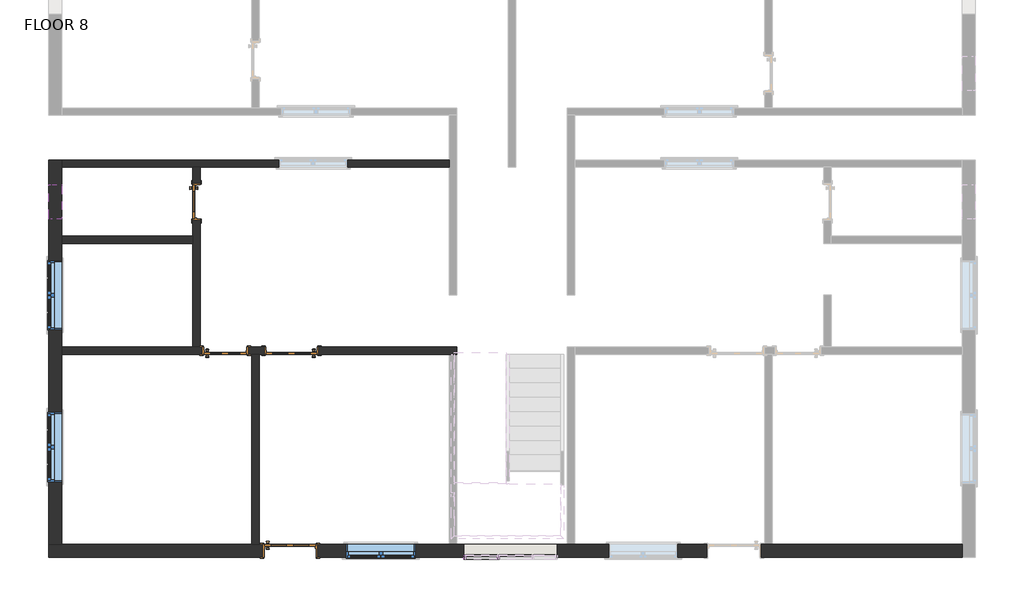
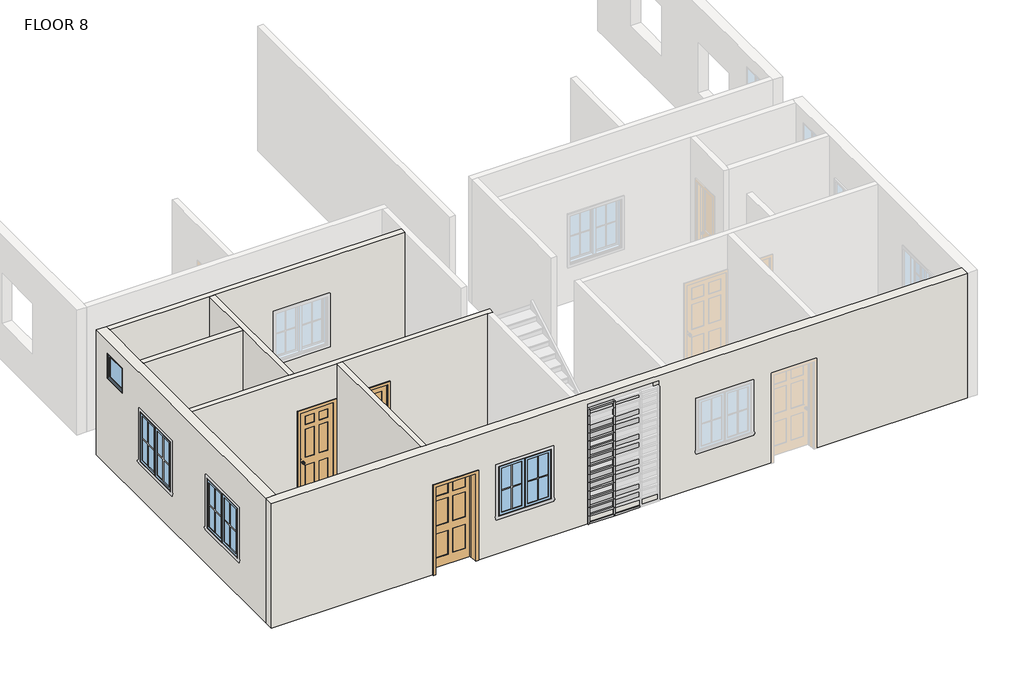
# One storey, part 1 of 4: 42 members, 20 plates, 7 walls, 4 doors, 4 windows.
"""IFC4 building model written with IfcOpenShell, lengths in millimetres."""

from ifc_helpers import new_model, si_unit, frame, origin, place, context, project, spatial, polyline, outline, extrude, faceted_brep, transform, mapped, element, save
from components import door_e337afa5, door_3b50870b, door_d86b6c54, door_03e3dfb5, member_56b223d9, member_a59c64b1, member_fa69921b, member_a67f877f, member_6a7c88b6, member_dc11c383, member_ff422208, system_panel_glazed_844a74e3, system_panel_glazed_a39216e9, system_panel_glazed_b3845325, system_panel_glazed_23b8b45c, system_panel_glazed_26c33eb0, system_panel_glazed_afc0885c, window_80340324, window_9200f5ac

model = new_model("IFC4")

# Units and contexts
model_context = context("Model", 3, world=origin())
ifc_project = project(units=[si_unit("LENGTHUNIT", "METRE", prefix="MILLI")], contexts=[model_context])

# Site, building, storey
site = spatial("IfcSite", under=ifc_project)
building = spatial("IfcBuilding", under=site)
storey = spatial("IfcBuildingStorey", under=building, Name="FLOOR 8", Elevation=12744.7725604)

# Doors
placement = place(None, origin())
door_shape = door_e337afa5(model_context)
element("IfcDoor", 1, ObjectType="Door-Interior-Single-2_Panel-Wood : 24\" x 84\"", at=placement, inside=storey, context=model_context, shape_type="MappedRepresentation", body=[
    mapped(door_shape, transform((-9830.0887331, -1548.6593836, 12744.7725604), x_axis=(0.0, -1.0, 0.0), y_axis=(1.0, 0.0, 0.0), z_axis=(0.0, 0.0, 1.0))),
])
door_2_shape = door_3b50870b(model_context)
element("IfcDoor", 2, ObjectType="Door-Interior-Single-6_Panel-Wood : 30\" x 84\"", at=placement, inside=storey, context=model_context, shape_type="MappedRepresentation", body=[
    mapped(door_2_shape, transform((-9318.9137331, -4180.7343836, 12744.7725604), x_axis=(1.0, 0.0, 0.0), y_axis=(0.0, 1.0, 0.0), z_axis=(0.0, 0.0, 1.0))),
])
door_3_shape = door_d86b6c54(model_context)
element("IfcDoor", 3, ObjectType="Door-Interior-Single-6_Panel-Wood : 36\" x 84\"", at=placement, inside=storey, context=model_context, shape_type="MappedRepresentation", body=[
    mapped(door_3_shape, transform((-8175.9137331, -7704.9843836, 12744.7725604), x_axis=(1.0, 0.0, 0.0), y_axis=(0.0, 1.0, 0.0), z_axis=(0.0, 0.0, 1.0))),
])
door_4_shape = door_03e3dfb5(model_context)
element("IfcDoor", 4, ObjectType="Door-Interior-Single-6_Panel-Wood : 36\" x 84\"", at=placement, inside=storey, context=model_context, shape_type="MappedRepresentation", body=[
    mapped(door_4_shape, transform((-8150.5137331, -4180.7343836, 12744.7725604), x_axis=(-1.0, 0.0, 0.0), y_axis=(0.0, -1.0, 0.0), z_axis=(0.0, 0.0, 1.0))),
])

# Members
member_shape = member_56b223d9(model_context)
element("IfcMember", 5, ObjectType="Rectangular Mullion : 1.5\" x 2.5\" rectangular", at=placement, inside=storey, context=model_context, shape_type="MappedRepresentation", body=[
    mapped(member_shape, transform((-4508.9003411, -7822.4593836, 12744.7725604), x_axis=(1.0, 0.0, 0.0), y_axis=(0.0, -1.0, 0.0), z_axis=(0.0, 0.0, -1.0))),
])
element("IfcMember", 6, ObjectType="Rectangular Mullion : 1.5\" x 2.5\" rectangular", at=placement, inside=storey, context=model_context, shape_type="MappedRepresentation", body=[
    mapped(member_shape, transform((-4508.9003411, -7822.4593836, 12947.9725604), x_axis=(1.0, 0.0, 0.0), y_axis=(0.0, -1.0, 0.0), z_axis=(0.0, 0.0, -1.0))),
])
element("IfcMember", 7, ObjectType="Rectangular Mullion : 1.5\" x 2.5\" rectangular", at=placement, inside=storey, context=model_context, shape_type="MappedRepresentation", body=[
    mapped(member_shape, transform((-4508.9003411, -7822.4593836, 13151.1725604), x_axis=(1.0, 0.0, 0.0), y_axis=(0.0, -1.0, 0.0), z_axis=(0.0, 0.0, -1.0))),
])
element("IfcMember", 8, ObjectType="Rectangular Mullion : 1.5\" x 2.5\" rectangular", at=placement, inside=storey, context=model_context, shape_type="MappedRepresentation", body=[
    mapped(member_shape, transform((-4508.9003411, -7822.4593836, 13354.3725604), x_axis=(1.0, 0.0, 0.0), y_axis=(0.0, -1.0, 0.0), z_axis=(0.0, 0.0, -1.0))),
])
element("IfcMember", 9, ObjectType="Rectangular Mullion : 1.5\" x 2.5\" rectangular", at=placement, inside=storey, context=model_context, shape_type="MappedRepresentation", body=[
    mapped(member_shape, transform((-4508.9003411, -7822.4593836, 13557.5725604), x_axis=(1.0, 0.0, 0.0), y_axis=(0.0, -1.0, 0.0), z_axis=(0.0, 0.0, -1.0))),
])
element("IfcMember", 10, ObjectType="Rectangular Mullion : 1.5\" x 2.5\" rectangular", at=placement, inside=storey, context=model_context, shape_type="MappedRepresentation", body=[
    mapped(member_shape, transform((-4508.9003411, -7822.4593836, 13760.7725604), x_axis=(1.0, 0.0, 0.0), y_axis=(0.0, -1.0, 0.0), z_axis=(0.0, 0.0, -1.0))),
])
element("IfcMember", 11, ObjectType="Rectangular Mullion : 1.5\" x 2.5\" rectangular", at=placement, inside=storey, context=model_context, shape_type="MappedRepresentation", body=[
    mapped(member_shape, transform((-4508.9003411, -7822.4593836, 13963.9725604), x_axis=(1.0, 0.0, 0.0), y_axis=(0.0, -1.0, 0.0), z_axis=(0.0, 0.0, -1.0))),
])
element("IfcMember", 12, ObjectType="Rectangular Mullion : 1.5\" x 2.5\" rectangular", at=placement, inside=storey, context=model_context, shape_type="MappedRepresentation", body=[
    mapped(member_shape, transform((-4508.9003411, -7822.4593836, 14167.1725604), x_axis=(1.0, 0.0, 0.0), y_axis=(0.0, -1.0, 0.0), z_axis=(0.0, 0.0, -1.0))),
])
element("IfcMember", 13, ObjectType="Rectangular Mullion : 1.5\" x 2.5\" rectangular", at=placement, inside=storey, context=model_context, shape_type="MappedRepresentation", body=[
    mapped(member_shape, transform((-4508.9003411, -7822.4593836, 14370.3725604), x_axis=(1.0, 0.0, 0.0), y_axis=(0.0, -1.0, 0.0), z_axis=(0.0, 0.0, -1.0))),
])
element("IfcMember", 14, ObjectType="Rectangular Mullion : 1.5\" x 2.5\" rectangular", at=placement, inside=storey, context=model_context, shape_type="MappedRepresentation", body=[
    mapped(member_shape, transform((-4508.9003411, -7822.4593836, 14573.5725604), x_axis=(1.0, 0.0, 0.0), y_axis=(0.0, -1.0, 0.0), z_axis=(0.0, 0.0, -1.0))),
])
element("IfcMember", 15, ObjectType="Rectangular Mullion : 1.5\" x 2.5\" rectangular", at=placement, inside=storey, context=model_context, shape_type="MappedRepresentation", body=[
    mapped(member_shape, transform((-4508.9003411, -7822.4593836, 14776.7725604), x_axis=(1.0, 0.0, 0.0), y_axis=(0.0, -1.0, 0.0), z_axis=(0.0, 0.0, -1.0))),
])
element("IfcMember", 16, ObjectType="Rectangular Mullion : 1.5\" x 2.5\" rectangular", at=placement, inside=storey, context=model_context, shape_type="MappedRepresentation", body=[
    mapped(member_shape, transform((-4508.9003411, -7822.4593836, 14979.9725604), x_axis=(1.0, 0.0, 0.0), y_axis=(0.0, -1.0, 0.0), z_axis=(0.0, 0.0, -1.0))),
])
element("IfcMember", 17, ObjectType="Rectangular Mullion : 1.5\" x 2.5\" rectangular", at=placement, inside=storey, context=model_context, shape_type="MappedRepresentation", body=[
    mapped(member_shape, transform((-4508.9003411, -7822.4593836, 15183.1725604), x_axis=(1.0, 0.0, 0.0), y_axis=(0.0, -1.0, 0.0), z_axis=(0.0, 0.0, -1.0))),
])
member_2_shape = member_a59c64b1(model_context)
element("IfcMember", 18, ObjectType="Rectangular Mullion : 1.5\" x 2.5\" rectangular", at=placement, inside=storey, context=model_context, shape_type="MappedRepresentation", body=[
    mapped(member_2_shape, transform((-4508.9003411, -7822.4593836, 15386.3725604), x_axis=(1.0, 0.0, 0.0), y_axis=(0.0, -1.0, 0.0), z_axis=(0.0, 0.0, -1.0))),
])
member_3_shape = member_fa69921b(model_context)
element("IfcMember", 19, ObjectType="Rectangular Mullion : 1.5\" x 2.5\" rectangular", at=placement, inside=storey, context=model_context, shape_type="MappedRepresentation", body=[
    mapped(member_3_shape, transform((-4527.9503411, -7822.4593836, 15552.1551755), x_axis=(0.0, 0.0, 1.0), y_axis=(0.0, -1.0, 0.0), z_axis=(1.0, 0.0, 0.0))),
])
element("IfcMember", 20, ObjectType="Rectangular Mullion : 1.5\" x 2.5\" rectangular", at=placement, inside=storey, context=model_context, shape_type="MappedRepresentation", body=[
    mapped(member_3_shape, transform((-5080.4003414, -7822.4593836, 12744.7725604), x_axis=(0.0, 0.0, -1.0), y_axis=(0.0, -1.0, 0.0), z_axis=(-1.0, 0.0, 0.0))),
])
member_4_shape = member_a67f877f(model_context)
element("IfcMember", 21, ObjectType="Rectangular Mullion : 1.5\" x 2.5\" rectangular", at=placement, inside=storey, context=model_context, shape_type="MappedRepresentation", body=[
    mapped(member_4_shape, transform((-4489.8503411, -7822.4593836, 12744.7725604), x_axis=(0.0, 0.0, -1.0), y_axis=(0.0, -1.0, 0.0), z_axis=(-1.0, 0.0, 0.0))),
])
member_5_shape = member_6a7c88b6(model_context)
element("IfcMember", 22, ObjectType="Rectangular Mullion : 1.5\" x 2.5\" rectangular", at=placement, inside=storey, context=model_context, shape_type="MappedRepresentation", body=[
    mapped(member_5_shape, transform((-4527.9503411, -7822.4593836, 12947.9725604), x_axis=(0.0, 0.0, 1.0), y_axis=(0.0, -1.0, 0.0), z_axis=(1.0, 0.0, 0.0))),
])
element("IfcMember", 23, ObjectType="Rectangular Mullion : 1.5\" x 2.5\" rectangular", at=placement, inside=storey, context=model_context, shape_type="MappedRepresentation", body=[
    mapped(member_5_shape, transform((-4527.9503411, -7822.4593836, 13151.1725604), x_axis=(0.0, 0.0, 1.0), y_axis=(0.0, -1.0, 0.0), z_axis=(1.0, 0.0, 0.0))),
])
element("IfcMember", 24, ObjectType="Rectangular Mullion : 1.5\" x 2.5\" rectangular", at=placement, inside=storey, context=model_context, shape_type="MappedRepresentation", body=[
    mapped(member_5_shape, transform((-4527.9503411, -7822.4593836, 13354.3725604), x_axis=(0.0, 0.0, 1.0), y_axis=(0.0, -1.0, 0.0), z_axis=(1.0, 0.0, 0.0))),
])
element("IfcMember", 25, ObjectType="Rectangular Mullion : 1.5\" x 2.5\" rectangular", at=placement, inside=storey, context=model_context, shape_type="MappedRepresentation", body=[
    mapped(member_5_shape, transform((-4527.9503411, -7822.4593836, 13557.5725604), x_axis=(0.0, 0.0, 1.0), y_axis=(0.0, -1.0, 0.0), z_axis=(1.0, 0.0, 0.0))),
])
element("IfcMember", 26, ObjectType="Rectangular Mullion : 1.5\" x 2.5\" rectangular", at=placement, inside=storey, context=model_context, shape_type="MappedRepresentation", body=[
    mapped(member_5_shape, transform((-4527.9503411, -7822.4593836, 13760.7725604), x_axis=(0.0, 0.0, 1.0), y_axis=(0.0, -1.0, 0.0), z_axis=(1.0, 0.0, 0.0))),
])
element("IfcMember", 27, ObjectType="Rectangular Mullion : 1.5\" x 2.5\" rectangular", at=placement, inside=storey, context=model_context, shape_type="MappedRepresentation", body=[
    mapped(member_5_shape, transform((-4527.9503411, -7822.4593836, 13963.9725604), x_axis=(0.0, 0.0, 1.0), y_axis=(0.0, -1.0, 0.0), z_axis=(1.0, 0.0, 0.0))),
])
element("IfcMember", 28, ObjectType="Rectangular Mullion : 1.5\" x 2.5\" rectangular", at=placement, inside=storey, context=model_context, shape_type="MappedRepresentation", body=[
    mapped(member_5_shape, transform((-4527.9503411, -7822.4593836, 14167.1725604), x_axis=(0.0, 0.0, 1.0), y_axis=(0.0, -1.0, 0.0), z_axis=(1.0, 0.0, 0.0))),
])
element("IfcMember", 29, ObjectType="Rectangular Mullion : 1.5\" x 2.5\" rectangular", at=placement, inside=storey, context=model_context, shape_type="MappedRepresentation", body=[
    mapped(member_5_shape, transform((-4527.9503411, -7822.4593836, 14370.3725604), x_axis=(0.0, 0.0, 1.0), y_axis=(0.0, -1.0, 0.0), z_axis=(1.0, 0.0, 0.0))),
])
element("IfcMember", 30, ObjectType="Rectangular Mullion : 1.5\" x 2.5\" rectangular", at=placement, inside=storey, context=model_context, shape_type="MappedRepresentation", body=[
    mapped(member_5_shape, transform((-4527.9503411, -7822.4593836, 14573.5725604), x_axis=(0.0, 0.0, 1.0), y_axis=(0.0, -1.0, 0.0), z_axis=(1.0, 0.0, 0.0))),
])
element("IfcMember", 31, ObjectType="Rectangular Mullion : 1.5\" x 2.5\" rectangular", at=placement, inside=storey, context=model_context, shape_type="MappedRepresentation", body=[
    mapped(member_5_shape, transform((-4527.9503411, -7822.4593836, 14776.7725604), x_axis=(0.0, 0.0, 1.0), y_axis=(0.0, -1.0, 0.0), z_axis=(1.0, 0.0, 0.0))),
])
element("IfcMember", 32, ObjectType="Rectangular Mullion : 1.5\" x 2.5\" rectangular", at=placement, inside=storey, context=model_context, shape_type="MappedRepresentation", body=[
    mapped(member_5_shape, transform((-4527.9503411, -7822.4593836, 14979.9725604), x_axis=(0.0, 0.0, 1.0), y_axis=(0.0, -1.0, 0.0), z_axis=(1.0, 0.0, 0.0))),
])
member_6_shape = member_dc11c383(model_context)
element("IfcMember", 33, ObjectType="Rectangular Mullion : 1.5\" x 2.5\" rectangular", at=placement, inside=storey, context=model_context, shape_type="MappedRepresentation", body=[
    mapped(member_6_shape, transform((-5118.5003414, -7822.4593836, 15552.1551755), x_axis=(-1.0, 0.0, 0.0), y_axis=(0.0, -1.0, 0.0), z_axis=(0.0, 0.0, 1.0))),
])
member_7_shape = member_ff422208(model_context)
element("IfcMember", 34, ObjectType="Rectangular Mullion : 1.5\" x 2.5\" rectangular", at=placement, inside=storey, context=model_context, shape_type="MappedRepresentation", body=[
    mapped(member_7_shape, transform((-5118.5003414, -7822.4593836, 12947.9725604), x_axis=(-1.0, 0.0, 0.0), y_axis=(0.0, -1.0, 0.0), z_axis=(0.0, 0.0, 1.0))),
])
element("IfcMember", 35, ObjectType="Rectangular Mullion : 1.5\" x 2.5\" rectangular", at=placement, inside=storey, context=model_context, shape_type="MappedRepresentation", body=[
    mapped(member_7_shape, transform((-5118.5003414, -7822.4593836, 13151.1725604), x_axis=(-1.0, 0.0, 0.0), y_axis=(0.0, -1.0, 0.0), z_axis=(0.0, 0.0, 1.0))),
])
element("IfcMember", 36, ObjectType="Rectangular Mullion : 1.5\" x 2.5\" rectangular", at=placement, inside=storey, context=model_context, shape_type="MappedRepresentation", body=[
    mapped(member_7_shape, transform((-5118.5003414, -7822.4593836, 13354.3725604), x_axis=(-1.0, 0.0, 0.0), y_axis=(0.0, -1.0, 0.0), z_axis=(0.0, 0.0, 1.0))),
])
element("IfcMember", 37, ObjectType="Rectangular Mullion : 1.5\" x 2.5\" rectangular", at=placement, inside=storey, context=model_context, shape_type="MappedRepresentation", body=[
    mapped(member_7_shape, transform((-5118.5003414, -7822.4593836, 13557.5725604), x_axis=(-1.0, 0.0, 0.0), y_axis=(0.0, -1.0, 0.0), z_axis=(0.0, 0.0, 1.0))),
])
element("IfcMember", 38, ObjectType="Rectangular Mullion : 1.5\" x 2.5\" rectangular", at=placement, inside=storey, context=model_context, shape_type="MappedRepresentation", body=[
    mapped(member_7_shape, transform((-5118.5003414, -7822.4593836, 13760.7725604), x_axis=(-1.0, 0.0, 0.0), y_axis=(0.0, -1.0, 0.0), z_axis=(0.0, 0.0, 1.0))),
])
element("IfcMember", 39, ObjectType="Rectangular Mullion : 1.5\" x 2.5\" rectangular", at=placement, inside=storey, context=model_context, shape_type="MappedRepresentation", body=[
    mapped(member_7_shape, transform((-5118.5003414, -7822.4593836, 13963.9725604), x_axis=(-1.0, 0.0, 0.0), y_axis=(0.0, -1.0, 0.0), z_axis=(0.0, 0.0, 1.0))),
])
element("IfcMember", 40, ObjectType="Rectangular Mullion : 1.5\" x 2.5\" rectangular", at=placement, inside=storey, context=model_context, shape_type="MappedRepresentation", body=[
    mapped(member_7_shape, transform((-5118.5003414, -7822.4593836, 14167.1725604), x_axis=(-1.0, 0.0, 0.0), y_axis=(0.0, -1.0, 0.0), z_axis=(0.0, 0.0, 1.0))),
])
element("IfcMember", 41, ObjectType="Rectangular Mullion : 1.5\" x 2.5\" rectangular", at=placement, inside=storey, context=model_context, shape_type="MappedRepresentation", body=[
    mapped(member_7_shape, transform((-5118.5003414, -7822.4593836, 14370.3725604), x_axis=(-1.0, 0.0, 0.0), y_axis=(0.0, -1.0, 0.0), z_axis=(0.0, 0.0, 1.0))),
])
element("IfcMember", 42, ObjectType="Rectangular Mullion : 1.5\" x 2.5\" rectangular", at=placement, inside=storey, context=model_context, shape_type="MappedRepresentation", body=[
    mapped(member_7_shape, transform((-5118.5003414, -7822.4593836, 14573.5725604), x_axis=(-1.0, 0.0, 0.0), y_axis=(0.0, -1.0, 0.0), z_axis=(0.0, 0.0, 1.0))),
])
element("IfcMember", 43, ObjectType="Rectangular Mullion : 1.5\" x 2.5\" rectangular", at=placement, inside=storey, context=model_context, shape_type="MappedRepresentation", body=[
    mapped(member_7_shape, transform((-5118.5003414, -7822.4593836, 14776.7725604), x_axis=(-1.0, 0.0, 0.0), y_axis=(0.0, -1.0, 0.0), z_axis=(0.0, 0.0, 1.0))),
])
element("IfcMember", 44, ObjectType="Rectangular Mullion : 1.5\" x 2.5\" rectangular", at=placement, inside=storey, context=model_context, shape_type="MappedRepresentation", body=[
    mapped(member_7_shape, transform((-5118.5003414, -7822.4593836, 14979.9725604), x_axis=(-1.0, 0.0, 0.0), y_axis=(0.0, -1.0, 0.0), z_axis=(0.0, 0.0, 1.0))),
])
element("IfcMember", 45, ObjectType="Rectangular Mullion : 1.5\" x 2.5\" rectangular", at=placement, inside=storey, context=model_context, shape_type="MappedRepresentation", body=[
    mapped(member_7_shape, transform((-5118.5003414, -7822.4593836, 15183.1725604), x_axis=(-1.0, 0.0, 0.0), y_axis=(0.0, -1.0, 0.0), z_axis=(0.0, 0.0, 1.0))),
])
element("IfcMember", 46, ObjectType="Rectangular Mullion : 1.5\" x 2.5\" rectangular", at=placement, inside=storey, context=model_context, shape_type="MappedRepresentation", body=[
    mapped(member_7_shape, transform((-5118.5003414, -7822.4593836, 15386.3725604), x_axis=(-1.0, 0.0, 0.0), y_axis=(0.0, -1.0, 0.0), z_axis=(0.0, 0.0, 1.0))),
])

# Plates
system_panel_glazed_shape = system_panel_glazed_844a74e3(model_context)
element("IfcPlate", 47, ObjectType="System Panel : Glazed", at=placement, inside=storey, context=model_context, shape_type="MappedRepresentation", body=[
    mapped(system_panel_glazed_shape, transform((-4804.1753412, -7822.4593836, 12782.8725604), x_axis=(1.0, 0.0, 0.0), y_axis=(0.0, 1.0, 0.0), z_axis=(0.0, 0.0, 1.0))),
])
system_panel_glazed_2_shape = system_panel_glazed_a39216e9(model_context)
element("IfcPlate", 48, ObjectType="System Panel : Glazed", at=placement, inside=storey, context=model_context, shape_type="MappedRepresentation", body=[
    mapped(system_panel_glazed_2_shape, transform((-4204.1003411, -7822.4593836, 12782.8725604), x_axis=(1.0, 0.0, 0.0), y_axis=(0.0, 1.0, 0.0), z_axis=(0.0, 0.0, 1.0))),
])
system_panel_glazed_3_shape = system_panel_glazed_b3845325(model_context)
element("IfcPlate", 49, ObjectType="System Panel : Glazed", at=placement, inside=storey, context=model_context, shape_type="MappedRepresentation", body=[
    mapped(system_panel_glazed_3_shape, transform((-4804.1753412, -7822.4593836, 12967.0225604), x_axis=(1.0, 0.0, 0.0), y_axis=(0.0, 1.0, 0.0), z_axis=(0.0, 0.0, 1.0))),
])
element("IfcPlate", 50, ObjectType="System Panel : Glazed", at=placement, inside=storey, context=model_context, shape_type="MappedRepresentation", body=[
    mapped(system_panel_glazed_3_shape, transform((-4804.1753412, -7822.4593836, 13170.2225604), x_axis=(1.0, 0.0, 0.0), y_axis=(0.0, 1.0, 0.0), z_axis=(0.0, 0.0, 1.0))),
])
element("IfcPlate", 51, ObjectType="System Panel : Glazed", at=placement, inside=storey, context=model_context, shape_type="MappedRepresentation", body=[
    mapped(system_panel_glazed_3_shape, transform((-4804.1753412, -7822.4593836, 13576.6225604), x_axis=(1.0, 0.0, 0.0), y_axis=(0.0, 1.0, 0.0), z_axis=(0.0, 0.0, 1.0))),
])
element("IfcPlate", 52, ObjectType="System Panel : Glazed", at=placement, inside=storey, context=model_context, shape_type="MappedRepresentation", body=[
    mapped(system_panel_glazed_3_shape, transform((-4804.1753412, -7822.4593836, 13779.8225604), x_axis=(1.0, 0.0, 0.0), y_axis=(0.0, 1.0, 0.0), z_axis=(0.0, 0.0, 1.0))),
])
element("IfcPlate", 53, ObjectType="System Panel : Glazed", at=placement, inside=storey, context=model_context, shape_type="MappedRepresentation", body=[
    mapped(system_panel_glazed_3_shape, transform((-4804.1753412, -7822.4593836, 14186.2225604), x_axis=(1.0, 0.0, 0.0), y_axis=(0.0, 1.0, 0.0), z_axis=(0.0, 0.0, 1.0))),
])
element("IfcPlate", 54, ObjectType="System Panel : Glazed", at=placement, inside=storey, context=model_context, shape_type="MappedRepresentation", body=[
    mapped(system_panel_glazed_3_shape, transform((-4804.1753412, -7822.4593836, 14389.4225604), x_axis=(1.0, 0.0, 0.0), y_axis=(0.0, 1.0, 0.0), z_axis=(0.0, 0.0, 1.0))),
])
element("IfcPlate", 55, ObjectType="System Panel : Glazed", at=placement, inside=storey, context=model_context, shape_type="MappedRepresentation", body=[
    mapped(system_panel_glazed_3_shape, transform((-4804.1753412, -7822.4593836, 14795.8225604), x_axis=(1.0, 0.0, 0.0), y_axis=(0.0, 1.0, 0.0), z_axis=(0.0, 0.0, 1.0))),
])
element("IfcPlate", 56, ObjectType="System Panel : Glazed", at=placement, inside=storey, context=model_context, shape_type="MappedRepresentation", body=[
    mapped(system_panel_glazed_3_shape, transform((-4804.1753412, -7822.4593836, 14999.0225604), x_axis=(1.0, 0.0, 0.0), y_axis=(0.0, 1.0, 0.0), z_axis=(0.0, 0.0, 1.0))),
])
system_panel_glazed_4_shape = system_panel_glazed_23b8b45c(model_context)
element("IfcPlate", 57, ObjectType="System Panel : Glazed", at=placement, inside=storey, context=model_context, shape_type="MappedRepresentation", body=[
    mapped(system_panel_glazed_4_shape, transform((-4204.1003411, -7822.4593836, 12967.0225604), x_axis=(1.0, 0.0, 0.0), y_axis=(0.0, 1.0, 0.0), z_axis=(0.0, 0.0, 1.0))),
])
element("IfcPlate", 58, ObjectType="System Panel : Glazed", at=placement, inside=storey, context=model_context, shape_type="MappedRepresentation", body=[
    mapped(system_panel_glazed_4_shape, transform((-4204.1003411, -7822.4593836, 13170.2225604), x_axis=(1.0, 0.0, 0.0), y_axis=(0.0, 1.0, 0.0), z_axis=(0.0, 0.0, 1.0))),
])
element("IfcPlate", 59, ObjectType="System Panel : Glazed", at=placement, inside=storey, context=model_context, shape_type="MappedRepresentation", body=[
    mapped(system_panel_glazed_4_shape, transform((-4204.1003411, -7822.4593836, 13576.6225604), x_axis=(1.0, 0.0, 0.0), y_axis=(0.0, 1.0, 0.0), z_axis=(0.0, 0.0, 1.0))),
])
element("IfcPlate", 60, ObjectType="System Panel : Glazed", at=placement, inside=storey, context=model_context, shape_type="MappedRepresentation", body=[
    mapped(system_panel_glazed_4_shape, transform((-4204.1003411, -7822.4593836, 13779.8225604), x_axis=(1.0, 0.0, 0.0), y_axis=(0.0, 1.0, 0.0), z_axis=(0.0, 0.0, 1.0))),
])
element("IfcPlate", 61, ObjectType="System Panel : Glazed", at=placement, inside=storey, context=model_context, shape_type="MappedRepresentation", body=[
    mapped(system_panel_glazed_4_shape, transform((-4204.1003411, -7822.4593836, 14186.2225604), x_axis=(1.0, 0.0, 0.0), y_axis=(0.0, 1.0, 0.0), z_axis=(0.0, 0.0, 1.0))),
])
element("IfcPlate", 62, ObjectType="System Panel : Glazed", at=placement, inside=storey, context=model_context, shape_type="MappedRepresentation", body=[
    mapped(system_panel_glazed_4_shape, transform((-4204.1003411, -7822.4593836, 14389.4225604), x_axis=(1.0, 0.0, 0.0), y_axis=(0.0, 1.0, 0.0), z_axis=(0.0, 0.0, 1.0))),
])
element("IfcPlate", 63, ObjectType="System Panel : Glazed", at=placement, inside=storey, context=model_context, shape_type="MappedRepresentation", body=[
    mapped(system_panel_glazed_4_shape, transform((-4204.1003411, -7822.4593836, 14795.8225604), x_axis=(1.0, 0.0, 0.0), y_axis=(0.0, 1.0, 0.0), z_axis=(0.0, 0.0, 1.0))),
])
element("IfcPlate", 64, ObjectType="System Panel : Glazed", at=placement, inside=storey, context=model_context, shape_type="MappedRepresentation", body=[
    mapped(system_panel_glazed_4_shape, transform((-4204.1003411, -7822.4593836, 14999.0225604), x_axis=(1.0, 0.0, 0.0), y_axis=(0.0, 1.0, 0.0), z_axis=(0.0, 0.0, 1.0))),
])
system_panel_glazed_5_shape = system_panel_glazed_26c33eb0(model_context)
element("IfcPlate", 65, ObjectType="System Panel : Glazed", at=placement, inside=storey, context=model_context, shape_type="MappedRepresentation", body=[
    mapped(system_panel_glazed_5_shape, transform((-4804.1753412, -7822.4593836, 15405.4225604), x_axis=(1.0, 0.0, 0.0), y_axis=(0.0, 1.0, 0.0), z_axis=(0.0, 0.0, 1.0))),
])
system_panel_glazed_6_shape = system_panel_glazed_afc0885c(model_context)
element("IfcPlate", 66, ObjectType="System Panel : Glazed", at=placement, inside=storey, context=model_context, shape_type="MappedRepresentation", body=[
    mapped(system_panel_glazed_6_shape, transform((-4204.1003411, -7822.4593836, 15405.4225604), x_axis=(1.0, 0.0, 0.0), y_axis=(0.0, 1.0, 0.0), z_axis=(0.0, 0.0, 1.0))),
])

# Walls
element("IfcWall", 67, ObjectType="Inner Wall 5\"", at=placement, inside=storey, context=model_context, shape_type="Brep", body=[
    faceted_brep([(-12201.8137331, -939.0593836, 12744.7725604), (-9890.4137331, -939.0593836, 12744.7725604), (-9763.4137331, -939.0593836, 12744.7725604), (-5369.2137331, -939.0593836, 12744.7725604), (-5369.2137331, -939.0593836, 15792.7725604), (-9763.4137331, -939.0593836, 15792.7725604), (-9890.4137331, -939.0593836, 15792.7725604), (-12201.8137331, -939.0593836, 15792.7725604), (-7159.9137331, -939.0593836, 14878.3725604), (-7159.9137331, -939.0593836, 13659.1725604), (-8379.1137331, -939.0593836, 13659.1725604), (-8379.1137331, -939.0593836, 14878.3725604), (-12201.8137331, -812.0593836, 12744.7725604), (-12201.8137331, -812.0593836, 15792.7725604), (-5369.2137331, -812.0593836, 15792.7725604), (-5369.2137331, -812.0593836, 12744.7725604), (-7159.9137331, -812.0593836, 14878.3725604), (-8379.1137331, -812.0593836, 14878.3725604), (-8379.1137331, -812.0593836, 13659.1725604), (-7159.9137331, -812.0593836, 13659.1725604)], [[[0, 1, 2, 3, 4, 5, 6, 7], [8, 9, 10, 11]], [[12, 13, 14, 15], [16, 17, 18, 19]], [[3, 2, 1, 0, 12, 15]], [[7, 6, 5, 4, 14, 13]], [[0, 7, 13, 12]], [[4, 3, 15, 14]], [[9, 8, 16, 19]], [[10, 9, 19, 18]], [[11, 10, 18, 17]], [[8, 11, 17, 16]]]),
])
element("IfcWall", 68, ObjectType="Inner Wall 5\"", at=placement, inside=storey, context=model_context, shape_type="SweptSolid", body=[
    extrude(outline(polyline([(-8722.0137331, -4241.0593836), (-8722.0137331, -7593.8593836), (-8849.0137331, -7593.8593836), (-8849.0137331, -4241.0593836), (-8722.0137331, -4241.0593836)])), frame((0.0, 0.0, 12744.7725604), z_axis=(0.0, 0.0, 1.0), x_axis=(1.0, 0.0, 0.0)), (0.0, 0.0, 1.0), 3048.0),
])
element("IfcWall", 69, ObjectType="Inner Wall 5\"", at=placement, inside=storey, context=model_context, shape_type="Brep", body=[
    faceted_brep([(-12201.8137331, -4114.0593836, 15792.7725604), (-9890.4137331, -4114.0593836, 15792.7725604), (-9763.4137331, -4114.0593836, 15792.7725604), (-5242.2137331, -4114.0593836, 15792.7725604), (-5242.2137331, -4114.0593836, 12744.7725604), (-7667.9137331, -4114.0593836, 12744.7725604), (-7667.9137331, -4114.0593836, 14903.7725604), (-8633.1137331, -4114.0593836, 14903.7725604), (-8633.1137331, -4114.0593836, 12744.7725604), (-8912.5137331, -4114.0593836, 12744.7725604), (-8912.5137331, -4114.0593836, 14903.7725604), (-9725.3137331, -4114.0593836, 14903.7725604), (-9725.3137331, -4114.0593836, 12744.7725604), (-9763.4137331, -4114.0593836, 12744.7725604), (-9890.4137331, -4114.0593836, 12744.7725604), (-12201.8137331, -4114.0593836, 12744.7725604), (-5242.2137331, -4241.0593836, 15792.7725604), (-5369.2137331, -4241.0593836, 15792.7725604), (-8722.0137331, -4241.0593836, 15792.7725604), (-8849.0137331, -4241.0593836, 15792.7725604), (-12201.8137331, -4241.0593836, 15792.7725604), (-12201.8137331, -4241.0593836, 12744.7725604), (-9725.3137331, -4241.0593836, 12744.7725604), (-9725.3137331, -4241.0593836, 14903.7725604), (-8912.5137331, -4241.0593836, 14903.7725604), (-8912.5137331, -4241.0593836, 12744.7725604), (-8849.0137331, -4241.0593836, 12744.7725604), (-8722.0137331, -4241.0593836, 12744.7725604), (-8633.1137331, -4241.0593836, 12744.7725604), (-8633.1137331, -4241.0593836, 14903.7725604), (-7667.9137331, -4241.0593836, 14903.7725604), (-7667.9137331, -4241.0593836, 12744.7725604), (-5369.2137331, -4241.0593836, 12744.7725604), (-5242.2137331, -4241.0593836, 12744.7725604)], [[[0, 1, 2, 3, 4, 5, 6, 7, 8, 9, 10, 11, 12, 13, 14, 15]], [[16, 17, 18, 19, 20, 21, 22, 23, 24, 25, 26, 27, 28, 29, 30, 31, 32, 33]], [[21, 15, 14, 13, 12, 22]], [[4, 33, 32, 31, 5]], [[25, 9, 8, 28, 27, 26]], [[3, 2, 1, 0, 20, 19, 18, 17, 16]], [[0, 15, 21, 20]], [[4, 3, 16, 33]], [[10, 9, 25, 24]], [[11, 10, 24, 23]], [[12, 11, 23, 22]], [[7, 29, 28, 8]], [[29, 7, 6, 30]], [[30, 6, 5, 31]]]),
])
element("IfcWall", 70, ObjectType="Inner Wall 5\"", at=placement, inside=storey, context=model_context, shape_type="Brep", body=[
    faceted_brep([(-9763.4137331, -939.0593836, 15792.7725604), (-9763.4137331, -4114.0593836, 15792.7725604), (-9763.4137331, -4114.0593836, 12744.7725604), (-9763.4137331, -1878.8593836, 12744.7725604), (-9763.4137331, -1878.8593836, 14903.7725604), (-9763.4137331, -1218.4593836, 14903.7725604), (-9763.4137331, -1218.4593836, 12744.7725604), (-9763.4137331, -939.0593836, 12744.7725604), (-9890.4137331, -4114.0593836, 15792.7725604), (-9890.4137331, -2285.2593836, 15792.7725604), (-9890.4137331, -2158.2593836, 15792.7725604), (-9890.4137331, -939.0593836, 15792.7725604), (-9890.4137331, -939.0593836, 12744.7725604), (-9890.4137331, -1218.4593836, 12744.7725604), (-9890.4137331, -1218.4593836, 14903.7725604), (-9890.4137331, -1878.8593836, 14903.7725604), (-9890.4137331, -1878.8593836, 12744.7725604), (-9890.4137331, -2158.2593836, 12744.7725604), (-9890.4137331, -2285.2593836, 12744.7725604), (-9890.4137331, -4114.0593836, 12744.7725604)], [[[0, 1, 2, 3, 4, 5, 6, 7]], [[8, 9, 10, 11, 12, 13, 14, 15, 16, 17, 18, 19]], [[2, 19, 18, 17, 16, 3]], [[12, 7, 6, 13]], [[1, 0, 11, 10, 9, 8]], [[2, 1, 8, 19]], [[0, 7, 12, 11]], [[15, 4, 3, 16]], [[4, 15, 14, 5]], [[5, 14, 13, 6]]]),
])
element("IfcWall", 71, ObjectType="Inner Wall 5\"", at=placement, inside=storey, context=model_context, shape_type="SweptSolid", body=[
    extrude(outline(polyline([(-12201.8137331, -2158.2593836), (-9890.4137331, -2158.2593836), (-9890.4137331, -2285.2593836), (-12201.8137331, -2285.2593836), (-12201.8137331, -2158.2593836)])), frame((0.0, 0.0, 12744.7725604), z_axis=(0.0, 0.0, 1.0), x_axis=(1.0, 0.0, 0.0)), (0.0, 0.0, 1.0), 3048.0),
])
element("IfcWall", 72, ObjectType="outer wall 9\"", at=placement, inside=storey, context=model_context, shape_type="Brep", body=[
    faceted_brep([(3673.1862669, -7822.4593836, 15792.7725604), (-12430.4137331, -7822.4593836, 15792.7725604), (-12430.4137331, -7822.4593836, 12744.7725604), (-8658.5137331, -7822.4593836, 12744.7725604), (-8658.5137331, -7822.4593836, 14903.7725604), (-7693.3137331, -7822.4593836, 14903.7725604), (-7693.3137331, -7822.4593836, 12744.7725604), (-835.3137331, -7822.4593836, 12744.7725604), (-835.3137331, -7822.4593836, 14903.7725604), (129.8862669, -7822.4593836, 14903.7725604), (129.8862669, -7822.4593836, 12744.7725604), (3673.1862669, -7822.4593836, 12744.7725604), (-2562.5137331, -7822.4593836, 14878.3725604), (-1343.3137331, -7822.4593836, 14878.3725604), (-1343.3137331, -7822.4593836, 13659.1725604), (-2562.5137331, -7822.4593836, 13659.1725604), (-7185.3137331, -7822.4593836, 14878.3725604), (-5966.1137331, -7822.4593836, 14878.3725604), (-5966.1137331, -7822.4593836, 13659.1725604), (-7185.3137331, -7822.4593836, 13659.1725604), (-5118.5003414, -7822.4593836, 15666.3657453), (-3466.9970483, -7822.4593836, 15666.3657453), (-3466.9970483, -7822.4593836, 12937.0392504), (-5118.5003414, -7822.4593836, 12937.0392504), (-12430.4137331, -7593.8593836, 15792.7725604), (-12201.8137331, -7593.8593836, 15792.7725604), (-8849.0137331, -7593.8593836, 15792.7725604), (-8722.0137331, -7593.8593836, 15792.7725604), (-5369.2137331, -7593.8593836, 15792.7725604), (-5242.2137331, -7593.8593836, 15792.7725604), (-3286.4137331, -7593.8593836, 15792.7725604), (-3159.4137331, -7593.8593836, 15792.7725604), (193.3862669, -7593.8593836, 15792.7725604), (320.3862669, -7593.8593836, 15792.7725604), (3673.1862669, -7593.8593836, 15792.7725604), (3673.1862669, -7593.8593836, 12744.7725604), (320.3862669, -7593.8593836, 12744.7725604), (193.3862669, -7593.8593836, 12744.7725604), (129.8862669, -7593.8593836, 12744.7725604), (129.8862669, -7593.8593836, 14903.7725604), (-835.3137331, -7593.8593836, 14903.7725604), (-835.3137331, -7593.8593836, 12744.7725604), (-3159.4137331, -7593.8593836, 12744.7725604), (-3286.4137331, -7593.8593836, 12744.7725604), (-5242.2137331, -7593.8593836, 12744.7725604), (-5369.2137331, -7593.8593836, 12744.7725604), (-7693.3137331, -7593.8593836, 12744.7725604), (-7693.3137331, -7593.8593836, 14903.7725604), (-8658.5137331, -7593.8593836, 14903.7725604), (-8658.5137331, -7593.8593836, 12744.7725604), (-8722.0137331, -7593.8593836, 12744.7725604), (-8849.0137331, -7593.8593836, 12744.7725604), (-12201.8137331, -7593.8593836, 12744.7725604), (-12430.4137331, -7593.8593836, 12744.7725604), (-2562.5137331, -7593.8593836, 14878.3725604), (-2562.5137331, -7593.8593836, 13659.1725604), (-1343.3137331, -7593.8593836, 13659.1725604), (-1343.3137331, -7593.8593836, 14878.3725604), (-7185.3137331, -7593.8593836, 14878.3725604), (-7185.3137331, -7593.8593836, 13659.1725604), (-5966.1137331, -7593.8593836, 13659.1725604), (-5966.1137331, -7593.8593836, 14878.3725604), (-3466.9970483, -7593.8593836, 15666.3657453), (-5118.5003414, -7593.8593836, 15666.3657453), (-5118.5003414, -7593.8593836, 12937.0392504), (-3466.9970483, -7593.8593836, 12937.0392504)], [[[0, 1, 2, 3, 4, 5, 6, 7, 8, 9, 10, 11], [12, 13, 14, 15], [16, 17, 18, 19], [20, 21, 22, 23]], [[24, 25, 26, 27, 28, 29, 30, 31, 32, 33, 34, 35, 36, 37, 38, 39, 40, 41, 42, 43, 44, 45, 46, 47, 48, 49, 50, 51, 52, 53], [54, 55, 56, 57], [58, 59, 60, 61], [62, 63, 64, 65]], [[2, 53, 52, 51, 50, 49, 3]], [[35, 11, 10, 38, 37, 36]], [[6, 46, 45, 44, 43, 42, 41, 7]], [[1, 0, 34, 33, 32, 31, 30, 29, 28, 27, 26, 25, 24]], [[2, 1, 24, 53]], [[0, 11, 35, 34]], [[5, 47, 46, 6]], [[47, 5, 4, 48]], [[48, 4, 3, 49]], [[40, 8, 7, 41]], [[8, 40, 39, 9]], [[9, 39, 38, 10]], [[55, 54, 12, 15]], [[56, 55, 15, 14]], [[57, 56, 14, 13]], [[54, 57, 13, 12]], [[59, 58, 16, 19]], [[60, 59, 19, 18]], [[61, 60, 18, 17]], [[58, 61, 17, 16]], [[20, 63, 62, 21]], [[22, 65, 64, 23]], [[63, 20, 23, 64]], [[21, 62, 65, 22]]]),
])
element("IfcWall", 73, ObjectType="outer wall 9\"", at=placement, inside=storey, context=model_context, shape_type="Brep", body=[
    faceted_brep([(-12430.4137331, -812.0593836, 12744.7725604), (-12430.4137331, -7593.8593836, 12744.7725604), (-12430.4137331, -7593.8593836, 15792.7725604), (-12430.4137331, -812.0593836, 15792.7725604), (-12430.4137331, -5269.7593836, 14878.3725604), (-12430.4137331, -6488.9593836, 14878.3725604), (-12430.4137331, -6488.9593836, 13659.1725604), (-12430.4137331, -5269.7593836, 13659.1725604), (-12430.4137331, -2590.0593836, 14878.3725604), (-12430.4137331, -3809.2593836, 14878.3725604), (-12430.4137331, -3809.2593836, 13659.1725604), (-12430.4137331, -2590.0593836, 13659.1725604), (-12430.4137331, -1243.8593836, 15487.9725604), (-12430.4137331, -1853.4593836, 15487.9725604), (-12430.4137331, -1853.4593836, 14878.3725604), (-12430.4137331, -1243.8593836, 14878.3725604), (-12201.8137331, -812.0593836, 12744.7725604), (-12201.8137331, -812.0593836, 15792.7725604), (-12201.8137331, -939.0593836, 15792.7725604), (-12201.8137331, -2158.2593836, 15792.7725604), (-12201.8137331, -2285.2593836, 15792.7725604), (-12201.8137331, -4114.0593836, 15792.7725604), (-12201.8137331, -4241.0593836, 15792.7725604), (-12201.8137331, -7593.8593836, 15792.7725604), (-12201.8137331, -7593.8593836, 12744.7725604), (-12201.8137331, -4241.0593836, 12744.7725604), (-12201.8137331, -4114.0593836, 12744.7725604), (-12201.8137331, -2285.2593836, 12744.7725604), (-12201.8137331, -2158.2593836, 12744.7725604), (-12201.8137331, -939.0593836, 12744.7725604), (-12201.8137331, -5269.7593836, 14878.3725604), (-12201.8137331, -5269.7593836, 13659.1725604), (-12201.8137331, -6488.9593836, 13659.1725604), (-12201.8137331, -6488.9593836, 14878.3725604), (-12201.8137331, -2590.0593836, 14878.3725604), (-12201.8137331, -2590.0593836, 13659.1725604), (-12201.8137331, -3809.2593836, 13659.1725604), (-12201.8137331, -3809.2593836, 14878.3725604), (-12201.8137331, -1243.8593836, 15487.9725604), (-12201.8137331, -1243.8593836, 14878.3725604), (-12201.8137331, -1853.4593836, 14878.3725604), (-12201.8137331, -1853.4593836, 15487.9725604)], [[[0, 1, 2, 3], [4, 5, 6, 7], [8, 9, 10, 11], [12, 13, 14, 15]], [[16, 17, 18, 19, 20, 21, 22, 23, 24, 25, 26, 27, 28, 29], [30, 31, 32, 33], [34, 35, 36, 37], [38, 39, 40, 41]], [[1, 0, 16, 29, 28, 27, 26, 25, 24]], [[3, 2, 23, 22, 21, 20, 19, 18, 17]], [[2, 1, 24, 23]], [[0, 3, 17, 16]], [[31, 30, 4, 7]], [[32, 31, 7, 6]], [[33, 32, 6, 5]], [[30, 33, 5, 4]], [[35, 34, 8, 11]], [[36, 35, 11, 10]], [[37, 36, 10, 9]], [[34, 37, 9, 8]], [[39, 38, 12, 15]], [[40, 39, 15, 14]], [[41, 40, 14, 13]], [[38, 41, 13, 12]]]),
])

# Windows
window_shape = window_80340324(model_context)
element("IfcWindow", 74, ObjectType="Fixed : 24\" x 24\"", at=placement, inside=storey, context=model_context, shape_type="MappedRepresentation", body=[
    mapped(window_shape, transform((-12316.1137331, -1510.5593836, 13963.9725604), x_axis=(0.0, 1.0, 0.0), y_axis=(-1.0, 0.0, 0.0), z_axis=(0.0, 0.0, 1.0))),
])
window_2_shape = window_9200f5ac(model_context)
element("IfcWindow", 75, ObjectType="Window-Casement-Double : 48\" x 48\"", at=placement, inside=storey, context=model_context, shape_type="MappedRepresentation", body=[
    mapped(window_2_shape, transform((-6575.7137331, -7708.1593836, 12744.7725604), x_axis=(-1.0, 0.0, 0.0), y_axis=(0.0, -1.0, 0.0), z_axis=(0.0, 0.0, 1.0))),
])
element("IfcWindow", 76, ObjectType="Window-Casement-Double : 48\" x 48\"", at=placement, inside=storey, context=model_context, shape_type="MappedRepresentation", body=[
    mapped(window_2_shape, transform((-12316.1137331, -5879.3593836, 12744.7725604), x_axis=(0.0, 1.0, 0.0), y_axis=(-1.0, 0.0, 0.0), z_axis=(0.0, 0.0, 1.0))),
])
element("IfcWindow", 77, ObjectType="Window-Casement-Double : 48\" x 48\"", at=placement, inside=storey, context=model_context, shape_type="MappedRepresentation", body=[
    mapped(window_2_shape, transform((-12316.1137331, -3199.6593836, 12744.7725604), x_axis=(0.0, 1.0, 0.0), y_axis=(-1.0, 0.0, 0.0), z_axis=(0.0, 0.0, 1.0))),
])

save(model, "model.ifc")

# Revit data of these elements
# Type "Door-Interior-Single-2_Panel-Wood : 24\" x 84\""
#   Type Mark = "10"
#   Assembly Code = "C1020300"
#   Analytic Construction = "Wooden"
#   Top Rail = 0' - 4 11/16"
#   Thickness = 0' - 1 3/8"
#   Thermal Resistance (R) = 2.5876 (h·ft²·°F)/BTU
#   Swing Angle [instance default] = 90.00°
#   Stiles = 0' - 4 3/4"
#   Rough Width = 2' - 2"
#   Rough Height = 7' - 1"
#   Lock Rail = 0' - 7 1/2"
#   Height = 7' - 0"
#   Width = 2' - 0"
#   Heat Transfer Coefficient (U) = 0.3865 BTU/(h·ft²·°F)
#   Bottom Rail = 0' - 9 1/8"
#   Trim Material = Cherry
#   Panel Material = Cherry
#   Frame Material = Cherry
#   Door Handle Material = Aluminum
#   Visual Light Transmittance = 0
#   Solar Heat Gain Coefficient = 0
#   Wall Closure = (empty or 0)
#   Function = (empty or 0)
# Type "Door-Interior-Single-6_Panel-Wood : 30\" x 84\""
#   Type Mark = "9"
#   Assembly Code = "C1020300"
#   Analytic Construction = "Wooden"
#   Top Rail = 0' - 4 11/16"
#   Top Panel = 0' - 8"
#   Thickness = 0' - 1 3/8"
#   Thermal Resistance (R) = 2.5876 (h·ft²·°F)/BTU
#   Swing Angle [instance default] = 90.00°
#   Stiles = 0' - 4 3/4"
#   Rough Width = 2' - 8"
#   Rough Height = 7' - 1"
#   Mullion = 0' - 4 1/2"
#   Lock Rail = 0' - 7 1/2"
#   Intermediate Rail = 0' - 4 1/2"
#   Height = 7' - 0"
#   Width = 2' - 6"
#   Heat Transfer Coefficient (U) = 0.3865 BTU/(h·ft²·°F)
#   Bottom Rail = 0' - 9 1/8"
#   Trim Material = Cherry
#   Panel Material = Cherry
#   Frame Material = Cherry
#   Door Handle Material = Aluminum
#   Visual Light Transmittance = 0
#   Solar Heat Gain Coefficient = 0
#   Wall Closure = (empty or 0)
#   Function = (empty or 0)
# Type "Door-Interior-Single-6_Panel-Wood : 36\" x 84\""
#   Type Mark = "8"
#   Assembly Code = "C1020300"
#   Analytic Construction = "Wooden"
#   Top Rail = 0' - 4 11/16"
#   Top Panel = 0' - 11"
#   Thickness = 0' - 1 3/8"
#   Thermal Resistance (R) = 2.5876 (h·ft²·°F)/BTU
#   Swing Angle [instance default] = 90.00°
#   Stiles = 0' - 4 3/4"
#   Rough Width = 3' - 2"
#   Rough Height = 7' - 1"
#   Mullion = 0' - 4 1/2"
#   Lock Rail = 0' - 7 1/2"
#   Intermediate Rail = 0' - 4 1/2"
#   Height = 7' - 0"
#   Width = 3' - 0"
#   Heat Transfer Coefficient (U) = 0.3865 BTU/(h·ft²·°F)
#   Bottom Rail = 0' - 9 1/8"
#   Trim Material = Cherry
#   Panel Material = Cherry
#   Frame Material = Cherry
#   Door Handle Material = Aluminum
#   Visual Light Transmittance = 0
#   Solar Heat Gain Coefficient = 0
#   Wall Closure = (empty or 0)
#   Function = (empty or 0)
# Type "Rectangular Mullion : 1.5\" x 2.5\" rectangular"
#   built-in parameter 1007304 = 0.208333 (stored number, unit not read)
#   built-in parameter 1007301 = 0.0625 (stored number, unit not read)
#   built-in parameter 1007300 = 0.0625 (stored number, unit not read)
# Type "System Panel : Glazed"
#   Construction Type Id = "GSP4R"
#   Analytic Construction = "1/8 in Pilkington single glazing"
#   Visual Light Transmittance = 0.9
#   Solar Heat Gain Coefficient = 0.86
#   Heat Transfer Coefficient (U) = 1.18115 BTU/(h·ft²·°F)
#   Define Thermal Properties by = 1
# Type "Inner Wall 5\""
#   Assembly Code = "B2010"
#   Layers, outside or top first: 0' - 5" "wall paint" (function 1)
# Type "outer wall 9\""
#   Assembly Code = "B2010"
#   Layers, outside or top first: 0' - 9" "wall paint" (function 1)
# Type "Fixed : 24\" x 24\""
#   Type Mark = "3"
#   Construction Type Id = "GSP4R"
#   Assembly Code = "B2020100"
#   Analytic Construction = "1/8 in Pilkington single glazing"
#   Visual Light Transmittance = 0.9
#   Solar Heat Gain Coefficient = 0.78
#   Heat Transfer Coefficient (U) = 0.6496 BTU/(h·ft²·°F)
#   Height = 2' - 0"
#   Default Sill Height = 3' - 0"
#   Width = 2' - 0"
#   Window Inset = 0' - 0 3/4"
#   Define Thermal Properties by = 1
#   Define Thermal Properties by = 1
#   Glass Pane Material = Glass
#   Sash Material = Sash
#   Wall Closure = (empty or 0)
# Type "Window-Casement-Double : 48\" x 48\""
#   Type Mark = "18"
#   Fire Rating = "0.5h"
#   Assembly Code = "B2020100"
#   Analytic Construction = "Double glazing - domestic"
#   Frame Extension [instance default] = 0' - 0 1/4"
#   Window Inset [instance default] = 0' - 0"
#   Wall Thickness [instance default] = 0' - 6"
#   Interior Wall Closure [instance default] = 0' - 2 1/4"
#   Half Width = 2' - 0"
#   Visual Light Transmittance = 0.81
#   Thermal Resistance (R) = 1.8146 (h·ft²·°F)/BTU
#   Solar Heat Gain Coefficient = 0.76
#   Rough Width = 4' - 0 1/2"
#   Rough Height = 4' - 0 1/2"
#   Height = 4' - 0"
#   Heat Transfer Coefficient (U) = 0.5511 BTU/(h·ft²·°F)
#   Exterior Wall Closure [instance default] = 0' - 1 1/4"
#   Extension Jamb [instance default] = 0' - 2 1/4"
#   Default Sill Height = 3' - 0"
#   Width = 4' - 0"
#   Muntin Visibility = yes
#   Interior Trim Visibility [instance default] = yes
#   Exterior Trim Visibility [instance default] = yes
#   Extension Jamb Visibility [instance default] = yes
#   Interior Trim Material = Wood - Stained
#   Muntin Pattern = Muntin Pattern_2x2 : Muntin Pattern_2x2
#   Interior Trim = Trim-Window-Interior-Flat : Picture Frame
#   Interior Frame Material = Wood - Stained
#   Glass Panel Material = Glass
#   Exterior Trim Material = Clad - White
#   Exterior Trim = Trim-Window-Exterior-Flat : with Sill
#   Exterior Frame Material = Clad - White
#   Wall Closure = (empty or 0)
# Element 1 (IfcDoor, "Door-Interior-Single-2_Panel-Wood : 24\" x 84\"")
#   Swing Angle = 90.00°
#   Phase Created = New Construction
#   Materials on its faces: "Cherry", "Aluminum"
# Element 2 (IfcDoor, "Door-Interior-Single-6_Panel-Wood : 30\" x 84\"")
#   Swing Angle = 90.00°
#   Phase Created = New Construction
#   Materials on its faces: "Cherry", "Aluminum"
# Elements 3, 4 (IfcDoor, "Door-Interior-Single-6_Panel-Wood : 36\" x 84\"")
#   Swing Angle = 90.00°
#   Phase Created = New Construction
#   Materials on its faces: "Cherry", "Aluminum"
# Elements 5, 6, 7, 8, 9, 10, 11, 12, 13, 14, 15, 16, 17, 18, 19, 20, 21, 22, 23, 24, 25, 26, 27, 28, 29, 30, 31, 32, 33, 34, 35, 36, 37, 38, 39, 40, 41, 42, 43, 44, 45, 46 (IfcMember, "Rectangular Mullion : 1.5\" x 2.5\" rectangular")
#   Phase Created = New Construction
#   Materials on its faces: "Aluminum"
# Elements 47, 48, 49, 50, 51, 52, 53, 54, 55, 56, 57, 58, 59, 60, 61, 62, 63, 64, 65, 66 (IfcPlate, "System Panel : Glazed")
#   Phase Created = New Construction
#   Materials on its faces: "Glass"
# Element 67 (IfcWall, "Inner Wall 5\"")
#   Top Offset = 0' - 0"
#   Base Offset = 0' - 0"
#   Unconnected Height = 10' - 0"
#   wall height = 10' - 0"
#   Phase Created = New Construction
#   Base Constraint = FLOOR 8
#   Materials on its faces: "wall paint", "Clad - White"
# Elements 68, 69, 70, 71 (IfcWall, "Inner Wall 5\"")
#   Top Offset = 0' - 0"
#   Base Offset = 0' - 0"
#   Unconnected Height = 10' - 0"
#   wall height = 10' - 0"
#   Phase Created = New Construction
#   Base Constraint = FLOOR 8
#   Materials on its faces: "wall paint"
# Elements 72, 73 (IfcWall, "outer wall 9\"")
#   Top Offset = 0' - 0"
#   Base Offset = 0' - 0"
#   Unconnected Height = 10' - 0"
#   wall height = 10' - 0"
#   Phase Created = New Construction
#   Base Constraint = FLOOR 8
#   Materials on its faces: "wall paint", "Clad - White"
# Element 74 (IfcWindow, "Fixed : 24\" x 24\"")
#   Mark = "182"
#   Phase Created = New Construction
#   Materials on its faces: "Sash", "Glass"
# Element 75 (IfcWindow, "Window-Casement-Double : 48\" x 48\"")
#   Mark = "173"
#   Window Inset = 0' - 0"
#   Interior Wall Closure = 0' - 2 1/4"
#   Frame Extension = 0' - 0 1/4"
#   Exterior Wall Closure = 0' - 1 1/4"
#   Interior Trim Visibility = yes
#   Exterior Trim Visibility = yes
#   Phase Created = New Construction
#   Materials on its faces: "Wood - Stained", "Glass", "Clad - White"
# Element 76 (IfcWindow, "Window-Casement-Double : 48\" x 48\"")
#   Mark = "174"
#   Window Inset = 0' - 0"
#   Interior Wall Closure = 0' - 2 1/4"
#   Frame Extension = 0' - 0 1/4"
#   Exterior Wall Closure = 0' - 1 1/4"
#   Interior Trim Visibility = yes
#   Exterior Trim Visibility = yes
#   Phase Created = New Construction
#   Materials on its faces: "Wood - Stained", "Glass", "Clad - White"
# Element 77 (IfcWindow, "Window-Casement-Double : 48\" x 48\"")
#   Mark = "175"
#   Window Inset = 0' - 0"
#   Interior Wall Closure = 0' - 2 1/4"
#   Frame Extension = 0' - 0 1/4"
#   Exterior Wall Closure = 0' - 1 1/4"
#   Interior Trim Visibility = yes
#   Exterior Trim Visibility = yes
#   Phase Created = New Construction
#   Materials on its faces: "Wood - Stained", "Glass", "Clad - White"
# Materials
#   "Cherry": class "Wood", colour RGB 226 177 128, transparency 0, Description = "Prunus Serotina", Cost = 0
#   "Aluminum": class "Metal", colour RGB 247 247 247, transparency 0, Description = "Aluminum 6061", Cost = 0
#   "wall paint": class "Generic", colour RGB 120 120 120, transparency 0, Cost = 0
#   "Glass": class "Glass", colour RGB 0 128 192, transparency 0.75, Description = "Soda Lime Glass", Cost = 0
#   "Sash": class "Wood", colour RGB 224 178 126, transparency 0, Cost = 0
#   "Wood - Stained": class "Wood", colour RGB 224 178 126, transparency 0, Cost = 0
#   "Clad - White": class "Wood", colour RGB 242 242 238, transparency 0, Cost = 0
